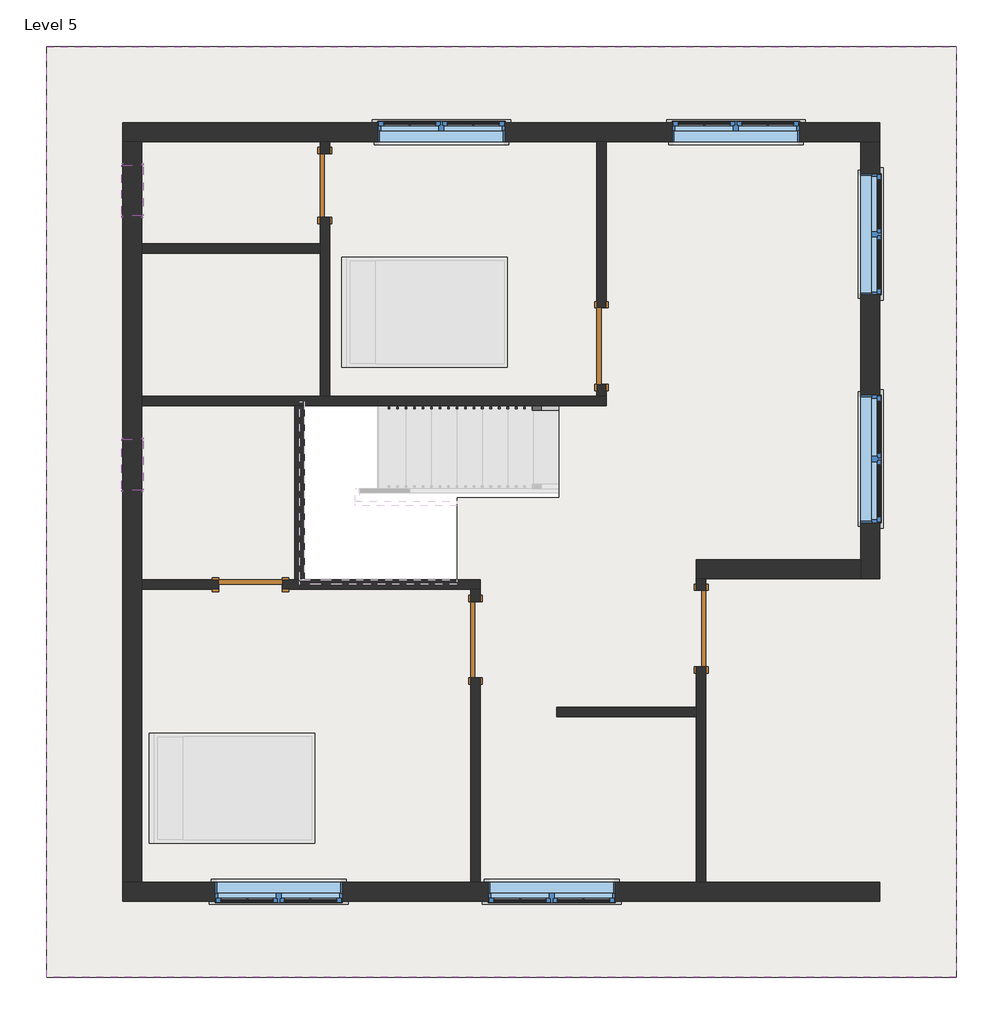
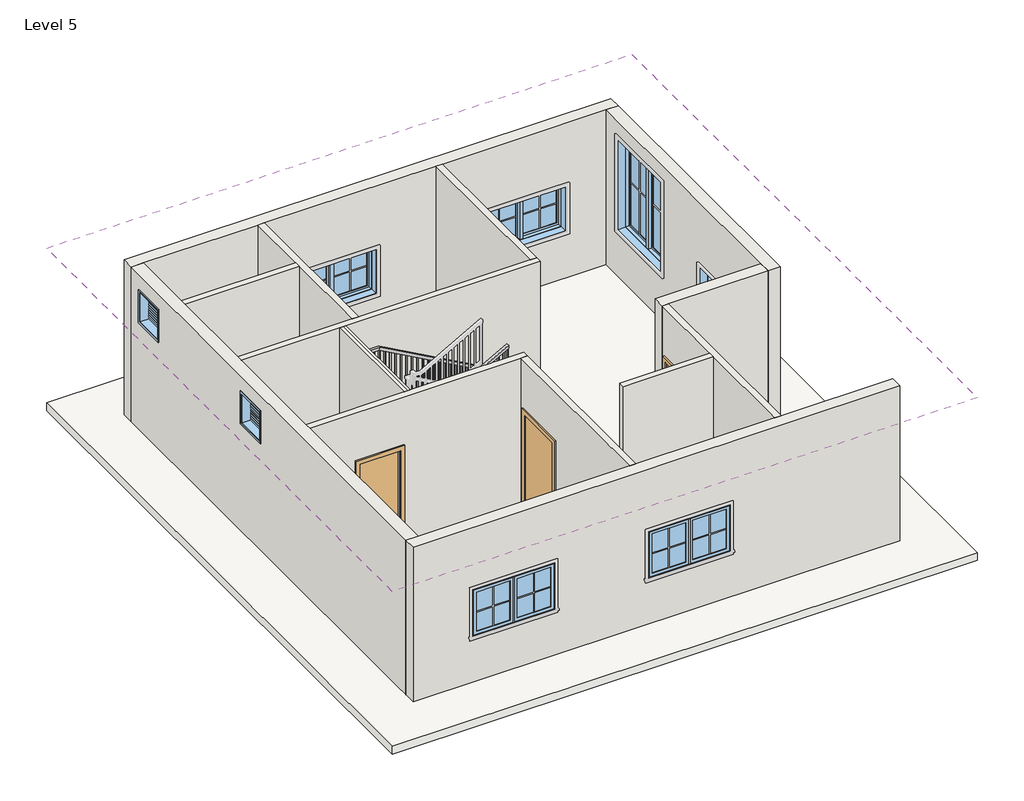
# One storey, part 1 of 2: 14 walls, 8 windows, 5 doors, 2 roofs, 1 railing.
"""IFC4 building model written with IfcOpenShell, lengths in millimetres."""

from ifc_helpers import new_model, si_unit, frame, origin, place, context, project, spatial, polyline, outline, extrude, faceted_brep, transform, mapped, element, save
from components import single_flush_3_17d80c48, single_flush_3_5e62189b, door_d8f5dbb5, window_9ac97e1a, window_c1d95f0f, window_f2d8fef0

model = new_model("IFC4")

# Units and contexts
model_context = context("Model", 3, world=origin())
ifc_project = project(units=[si_unit("LENGTHUNIT", "METRE", prefix="MILLI")], contexts=[model_context])

# Site, building, storey
site = spatial("IfcSite", under=ifc_project)
building = spatial("IfcBuilding", under=site)
storey = spatial("IfcBuildingStorey", under=building, Name="Level 5", Elevation=12649.2)

# Doors
placement = place(None, origin())
single_flush_3_shape = single_flush_3_17d80c48(model_context)
element("IfcDoor", 1, ObjectType="Single-Flush : 3'", at=placement, inside=storey, context=model_context, shape_type="MappedRepresentation", body=[
    mapped(single_flush_3_shape, transform((-1566.5130704, -2143.0042021, 12649.2), x_axis=(0.0, 1.0, 0.0), y_axis=(-1.0, 0.0, 0.0), z_axis=(0.0, 0.0, 1.0))),
])
single_flush_3_2_shape = single_flush_3_5e62189b(model_context)
element("IfcDoor", 2, ObjectType="Single-Flush : 3'", at=placement, inside=storey, context=model_context, shape_type="MappedRepresentation", body=[
    mapped(single_flush_3_2_shape, transform((1138.5869296, -2009.6542021, 12649.2), x_axis=(0.0, 1.0, 0.0), y_axis=(-1.0, 0.0, 0.0), z_axis=(0.0, 0.0, 1.0))),
])
element("IfcDoor", 3, ObjectType="Single-Flush : 3'", at=placement, inside=storey, context=model_context, shape_type="MappedRepresentation", body=[
    mapped(single_flush_3_2_shape, transform((-55.2130704, 1374.8957979, 12649.2), x_axis=(0.0, -1.0, 0.0), y_axis=(1.0, 0.0, 0.0), z_axis=(0.0, 0.0, 1.0))),
])
door_shape = door_d8f5dbb5(model_context)
element("IfcDoor", 4, ObjectType="Single-Flush : DOOR 2'6\"", at=placement, inside=storey, context=model_context, shape_type="MappedRepresentation", body=[
    mapped(door_shape, transform((-3369.9130704, 3298.9457979, 12649.2), x_axis=(0.0, 1.0, 0.0), y_axis=(-1.0, 0.0, 0.0), z_axis=(0.0, 0.0, 1.0))),
])
element("IfcDoor", 5, ObjectType="Single-Flush : DOOR 2'6\"", at=placement, inside=storey, context=model_context, shape_type="MappedRepresentation", body=[
    mapped(door_shape, transform((-4258.9130704, -1482.6042021, 12649.2), x_axis=(1.0, 0.0, 0.0), y_axis=(0.0, 1.0, 0.0), z_axis=(0.0, 0.0, 1.0))),
])

# Railing
element("IfcRailing", 6, ObjectType="Handrail - Rectangular", at=placement, inside=storey, context=model_context, shape_type="SolidModel", body=[
    faceted_brep([(-569.5630704, 606.5457979, 13732.9333333), (-569.5630704, 606.5457979, 13674.820221), (-569.5630704, 657.3457979, 13674.820221), (-569.5630704, 657.3457979, 13732.9333333), (-3007.9630704, 606.5457979, 15087.6), (-3021.1266727, 606.5457979, 15036.8), (-3021.1266727, 657.3457979, 15036.8), (-3007.9630704, 657.3457979, 15087.6), (-3566.7630704, 606.5457979, 15087.6), (-3566.7630704, 606.5457979, 15036.8), (-3617.5630704, 657.3457979, 15036.8), (-3617.5630704, 657.3457979, 15087.6), (-3566.7630704, -1374.6542021, 15087.6), (-3566.7630704, -1374.6542021, 15036.8), (-3617.5630704, -1425.4542021, 15036.8), (-3617.5630704, -1425.4542021, 15087.6), (-3312.7630704, -1374.6542021, 15087.6), (-3299.5994682, -1374.6542021, 15036.8), (-3299.5994682, -1425.4542021, 15036.8), (-3312.7630704, -1425.4542021, 15087.6), (-1788.7630704, -1374.6542021, 15934.2666667), (-1788.7630704, -1425.4542021, 15934.2666667), (-1788.7630704, -1425.4542021, 15876.1535543), (-1788.7630704, -1374.6542021, 15876.1535543)], [[[0, 1, 2, 3]], [[1, 0, 4, 5]], [[2, 1, 5, 6]], [[3, 2, 6, 7]], [[0, 3, 7, 4]], [[5, 4, 8, 9]], [[6, 5, 9, 10]], [[7, 6, 10, 11]], [[4, 7, 11, 8]], [[9, 8, 12, 13]], [[10, 9, 13, 14]], [[11, 10, 14, 15]], [[8, 11, 15, 12]], [[13, 12, 16, 17]], [[14, 13, 17, 18]], [[15, 14, 18, 19]], [[12, 15, 19, 16]], [[20, 21, 22, 23]], [[17, 16, 20, 23]], [[18, 17, 23, 22]], [[19, 18, 22, 21]], [[16, 19, 21, 20]]]),
    extrude(outline(polyline([(15839.1118876, -1855.4380704), (15828.5285543, -1874.4880704), (14850.5333333, -1874.4880704), (14850.5333333, -1855.4380704), (15839.1118876, -1855.4380704)])), frame((0.0, -1409.5792021, 0.0), z_axis=(0.0, 1.0, 0.0), x_axis=(0.0, 0.0, 1.0)), (0.0, 0.0, 1.0), 19.05),
    extrude(outline(polyline([(15782.6674432, -1957.0380704), (15772.0841099, -1976.0880704), (14850.5333333, -1976.0880704), (14850.5333333, -1957.0380704), (15782.6674432, -1957.0380704)])), frame((0.0, -1409.5792021, 0.0), z_axis=(0.0, 1.0, 0.0), x_axis=(0.0, 0.0, 1.0)), (0.0, 0.0, 1.0), 19.05),
    extrude(outline(polyline([(15726.2229988, -2058.6380704), (15715.6396654, -2077.6880704), (14850.5333333, -2077.6880704), (14850.5333333, -2058.6380704), (15726.2229988, -2058.6380704)])), frame((0.0, -1409.5792021, 0.0), z_axis=(0.0, 1.0, 0.0), x_axis=(0.0, 0.0, 1.0)), (0.0, 0.0, 1.0), 19.05),
    extrude(outline(polyline([(15669.7785543, -2160.2380704), (15659.195221, -2179.2880704), (14681.2, -2179.2880704), (14681.2, -2160.2380704), (15669.7785543, -2160.2380704)])), frame((0.0, -1409.5792021, 0.0), z_axis=(0.0, 1.0, 0.0), x_axis=(0.0, 0.0, 1.0)), (0.0, 0.0, 1.0), 19.05),
    extrude(outline(polyline([(15613.3341099, -2261.8380704), (15602.7507765, -2280.8880704), (14681.2, -2280.8880704), (14681.2, -2261.8380704), (15613.3341099, -2261.8380704)])), frame((0.0, -1409.5792021, 0.0), z_axis=(0.0, 1.0, 0.0), x_axis=(0.0, 0.0, 1.0)), (0.0, 0.0, 1.0), 19.05),
    extrude(outline(polyline([(15556.8896654, -2363.4380704), (15546.3063321, -2382.4880704), (14681.2, -2382.4880704), (14681.2, -2363.4380704), (15556.8896654, -2363.4380704)])), frame((0.0, -1409.5792021, 0.0), z_axis=(0.0, 1.0, 0.0), x_axis=(0.0, 0.0, 1.0)), (0.0, 0.0, 1.0), 19.05),
    extrude(outline(polyline([(15500.445221, -2465.0380704), (15489.8618876, -2484.0880704), (14511.8666667, -2484.0880704), (14511.8666667, -2465.0380704), (15500.445221, -2465.0380704)])), frame((0.0, -1409.5792021, 0.0), z_axis=(0.0, 1.0, 0.0), x_axis=(0.0, 0.0, 1.0)), (0.0, 0.0, 1.0), 19.05),
    extrude(outline(polyline([(15444.0007765, -2566.6380704), (15433.4174432, -2585.6880704), (14511.8666667, -2585.6880704), (14511.8666667, -2566.6380704), (15444.0007765, -2566.6380704)])), frame((0.0, -1409.5792021, 0.0), z_axis=(0.0, 1.0, 0.0), x_axis=(0.0, 0.0, 1.0)), (0.0, 0.0, 1.0), 19.05),
    extrude(outline(polyline([(15387.5563321, -2668.2380704), (15376.9729988, -2687.2880704), (14511.8666667, -2687.2880704), (14511.8666667, -2668.2380704), (15387.5563321, -2668.2380704)])), frame((0.0, -1409.5792021, 0.0), z_axis=(0.0, 1.0, 0.0), x_axis=(0.0, 0.0, 1.0)), (0.0, 0.0, 1.0), 19.05),
    extrude(outline(polyline([(15331.1118876, -2769.8380704), (15320.5285543, -2788.8880704), (14342.5333333, -2788.8880704), (14342.5333333, -2769.8380704), (15331.1118876, -2769.8380704)])), frame((0.0, -1409.5792021, 0.0), z_axis=(0.0, 1.0, 0.0), x_axis=(0.0, 0.0, 1.0)), (0.0, 0.0, 1.0), 19.05),
    extrude(outline(polyline([(15274.6674432, -2871.4380704), (15264.0841099, -2890.4880704), (14342.5333333, -2890.4880704), (14342.5333333, -2871.4380704), (15274.6674432, -2871.4380704)])), frame((0.0, -1409.5792021, 0.0), z_axis=(0.0, 1.0, 0.0), x_axis=(0.0, 0.0, 1.0)), (0.0, 0.0, 1.0), 19.05),
    extrude(outline(polyline([(15218.2229988, -2973.0380704), (15207.6396654, -2992.0880704), (14342.5333333, -2992.0880704), (14342.5333333, -2973.0380704), (15218.2229988, -2973.0380704)])), frame((0.0, -1409.5792021, 0.0), z_axis=(0.0, 1.0, 0.0), x_axis=(0.0, 0.0, 1.0)), (0.0, 0.0, 1.0), 19.05),
    extrude(outline(polyline([(15161.7785543, -3074.6380704), (15151.195221, -3093.6880704), (14173.2, -3093.6880704), (14173.2, -3074.6380704), (15161.7785543, -3074.6380704)])), frame((0.0, -1409.5792021, 0.0), z_axis=(0.0, 1.0, 0.0), x_axis=(0.0, 0.0, 1.0)), (0.0, 0.0, 1.0), 19.05),
    extrude(outline(polyline([(15105.3341099, -3176.2380704), (15094.7507765, -3195.2880704), (14173.2, -3195.2880704), (14173.2, -3176.2380704), (15105.3341099, -3176.2380704)])), frame((0.0, -1409.5792021, 0.0), z_axis=(0.0, 1.0, 0.0), x_axis=(0.0, 0.0, 1.0)), (0.0, 0.0, 1.0), 19.05),
    extrude(outline(polyline([(15048.8896654, -3277.8380704), (15038.3063321, -3296.8880704), (14173.2, -3296.8880704), (14173.2, -3277.8380704), (15048.8896654, -3277.8380704)])), frame((0.0, -1409.5792021, 0.0), z_axis=(0.0, 1.0, 0.0), x_axis=(0.0, 0.0, 1.0)), (0.0, 0.0, 1.0), 19.05),
    extrude(outline(polyline([(-3398.4880704, -1409.5792021), (-3398.4880704, -1390.5292021), (-3379.4380704, -1390.5292021), (-3379.4380704, -1409.5792021), (-3398.4880704, -1409.5792021)])), frame((0.0, 0.0, 14173.2), z_axis=(0.0, 0.0, 1.0), x_axis=(1.0, 0.0, 0.0)), (0.0, 0.0, 1.0), 863.6),
    extrude(outline(polyline([(-3500.0880704, -1409.5792021), (-3500.0880704, -1390.5292021), (-3481.0380704, -1390.5292021), (-3481.0380704, -1409.5792021), (-3500.0880704, -1409.5792021)])), frame((0.0, 0.0, 14173.2), z_axis=(0.0, 0.0, 1.0), x_axis=(1.0, 0.0, 0.0)), (0.0, 0.0, 1.0), 863.6),
    extrude(outline(polyline([(-3601.6880704, -1288.9292021), (-3582.6380704, -1288.9292021), (-3582.6380704, -1307.9792021), (-3601.6880704, -1307.9792021), (-3601.6880704, -1288.9292021)])), frame((0.0, 0.0, 14173.2), z_axis=(0.0, 0.0, 1.0), x_axis=(1.0, 0.0, 0.0)), (0.0, 0.0, 1.0), 863.6),
    extrude(outline(polyline([(-3601.6880704, -1187.3292021), (-3582.6380704, -1187.3292021), (-3582.6380704, -1206.3792021), (-3601.6880704, -1206.3792021), (-3601.6880704, -1187.3292021)])), frame((0.0, 0.0, 14173.2), z_axis=(0.0, 0.0, 1.0), x_axis=(1.0, 0.0, 0.0)), (0.0, 0.0, 1.0), 863.6),
    extrude(outline(polyline([(-3601.6880704, -1085.7292021), (-3582.6380704, -1085.7292021), (-3582.6380704, -1104.7792021), (-3601.6880704, -1104.7792021), (-3601.6880704, -1085.7292021)])), frame((0.0, 0.0, 14173.2), z_axis=(0.0, 0.0, 1.0), x_axis=(1.0, 0.0, 0.0)), (0.0, 0.0, 1.0), 863.6),
    extrude(outline(polyline([(-3601.6880704, -984.1292021), (-3582.6380704, -984.1292021), (-3582.6380704, -1003.1792021), (-3601.6880704, -1003.1792021), (-3601.6880704, -984.1292021)])), frame((0.0, 0.0, 14173.2), z_axis=(0.0, 0.0, 1.0), x_axis=(1.0, 0.0, 0.0)), (0.0, 0.0, 1.0), 863.6),
    extrude(outline(polyline([(-3601.6880704, -882.5292021), (-3582.6380704, -882.5292021), (-3582.6380704, -901.5792021), (-3601.6880704, -901.5792021), (-3601.6880704, -882.5292021)])), frame((0.0, 0.0, 14173.2), z_axis=(0.0, 0.0, 1.0), x_axis=(1.0, 0.0, 0.0)), (0.0, 0.0, 1.0), 863.6),
    extrude(outline(polyline([(-3601.6880704, -780.9292021), (-3582.6380704, -780.9292021), (-3582.6380704, -799.9792021), (-3601.6880704, -799.9792021), (-3601.6880704, -780.9292021)])), frame((0.0, 0.0, 14173.2), z_axis=(0.0, 0.0, 1.0), x_axis=(1.0, 0.0, 0.0)), (0.0, 0.0, 1.0), 863.6),
    extrude(outline(polyline([(-3601.6880704, -679.3292021), (-3582.6380704, -679.3292021), (-3582.6380704, -698.3792021), (-3601.6880704, -698.3792021), (-3601.6880704, -679.3292021)])), frame((0.0, 0.0, 14173.2), z_axis=(0.0, 0.0, 1.0), x_axis=(1.0, 0.0, 0.0)), (0.0, 0.0, 1.0), 863.6),
    extrude(outline(polyline([(-3601.6880704, -577.7292021), (-3582.6380704, -577.7292021), (-3582.6380704, -596.7792021), (-3601.6880704, -596.7792021), (-3601.6880704, -577.7292021)])), frame((0.0, 0.0, 14173.2), z_axis=(0.0, 0.0, 1.0), x_axis=(1.0, 0.0, 0.0)), (0.0, 0.0, 1.0), 863.6),
    extrude(outline(polyline([(-3601.6880704, -476.1292021), (-3582.6380704, -476.1292021), (-3582.6380704, -495.1792021), (-3601.6880704, -495.1792021), (-3601.6880704, -476.1292021)])), frame((0.0, 0.0, 14173.2), z_axis=(0.0, 0.0, 1.0), x_axis=(1.0, 0.0, 0.0)), (0.0, 0.0, 1.0), 863.6),
    extrude(outline(polyline([(-3601.6880704, -374.5292021), (-3582.6380704, -374.5292021), (-3582.6380704, -393.5792021), (-3601.6880704, -393.5792021), (-3601.6880704, -374.5292021)])), frame((0.0, 0.0, 14173.2), z_axis=(0.0, 0.0, 1.0), x_axis=(1.0, 0.0, 0.0)), (0.0, 0.0, 1.0), 863.6),
    extrude(outline(polyline([(-3601.6880704, -272.9292021), (-3582.6380704, -272.9292021), (-3582.6380704, -291.9792021), (-3601.6880704, -291.9792021), (-3601.6880704, -272.9292021)])), frame((0.0, 0.0, 14173.2), z_axis=(0.0, 0.0, 1.0), x_axis=(1.0, 0.0, 0.0)), (0.0, 0.0, 1.0), 863.6),
    extrude(outline(polyline([(-3601.6880704, -171.3292021), (-3582.6380704, -171.3292021), (-3582.6380704, -190.3792021), (-3601.6880704, -190.3792021), (-3601.6880704, -171.3292021)])), frame((0.0, 0.0, 14173.2), z_axis=(0.0, 0.0, 1.0), x_axis=(1.0, 0.0, 0.0)), (0.0, 0.0, 1.0), 863.6),
    extrude(outline(polyline([(-3601.6880704, -69.7292021), (-3582.6380704, -69.7292021), (-3582.6380704, -88.7792021), (-3601.6880704, -88.7792021), (-3601.6880704, -69.7292021)])), frame((0.0, 0.0, 14173.2), z_axis=(0.0, 0.0, 1.0), x_axis=(1.0, 0.0, 0.0)), (0.0, 0.0, 1.0), 863.6),
    extrude(outline(polyline([(-3601.6880704, 31.8707979), (-3582.6380704, 31.8707979), (-3582.6380704, 12.8207979), (-3601.6880704, 12.8207979), (-3601.6880704, 31.8707979)])), frame((0.0, 0.0, 14173.2), z_axis=(0.0, 0.0, 1.0), x_axis=(1.0, 0.0, 0.0)), (0.0, 0.0, 1.0), 863.6),
    extrude(outline(polyline([(-3601.6880704, 133.4707979), (-3582.6380704, 133.4707979), (-3582.6380704, 114.4207979), (-3601.6880704, 114.4207979), (-3601.6880704, 133.4707979)])), frame((0.0, 0.0, 14173.2), z_axis=(0.0, 0.0, 1.0), x_axis=(1.0, 0.0, 0.0)), (0.0, 0.0, 1.0), 863.6),
    extrude(outline(polyline([(-3601.6880704, 235.0707979), (-3582.6380704, 235.0707979), (-3582.6380704, 216.0207979), (-3601.6880704, 216.0207979), (-3601.6880704, 235.0707979)])), frame((0.0, 0.0, 14173.2), z_axis=(0.0, 0.0, 1.0), x_axis=(1.0, 0.0, 0.0)), (0.0, 0.0, 1.0), 863.6),
    extrude(outline(polyline([(-3601.6880704, 336.6707979), (-3582.6380704, 336.6707979), (-3582.6380704, 317.6207979), (-3601.6880704, 317.6207979), (-3601.6880704, 336.6707979)])), frame((0.0, 0.0, 14173.2), z_axis=(0.0, 0.0, 1.0), x_axis=(1.0, 0.0, 0.0)), (0.0, 0.0, 1.0), 863.6),
    extrude(outline(polyline([(-3601.6880704, 438.2707979), (-3582.6380704, 438.2707979), (-3582.6380704, 419.2207979), (-3601.6880704, 419.2207979), (-3601.6880704, 438.2707979)])), frame((0.0, 0.0, 14173.2), z_axis=(0.0, 0.0, 1.0), x_axis=(1.0, 0.0, 0.0)), (0.0, 0.0, 1.0), 863.6),
    extrude(outline(polyline([(-3601.6880704, 539.8707979), (-3582.6380704, 539.8707979), (-3582.6380704, 520.8207979), (-3601.6880704, 520.8207979), (-3601.6880704, 539.8707979)])), frame((0.0, 0.0, 14173.2), z_axis=(0.0, 0.0, 1.0), x_axis=(1.0, 0.0, 0.0)), (0.0, 0.0, 1.0), 863.6),
    extrude(outline(polyline([(-3506.4380704, 641.4707979), (-3506.4380704, 622.4207979), (-3525.4880704, 622.4207979), (-3525.4880704, 641.4707979), (-3506.4380704, 641.4707979)])), frame((0.0, 0.0, 14173.2), z_axis=(0.0, 0.0, 1.0), x_axis=(1.0, 0.0, 0.0)), (0.0, 0.0, 1.0), 863.6),
    extrude(outline(polyline([(-3404.8380704, 641.4707979), (-3404.8380704, 622.4207979), (-3423.8880704, 622.4207979), (-3423.8880704, 641.4707979), (-3404.8380704, 641.4707979)])), frame((0.0, 0.0, 14173.2), z_axis=(0.0, 0.0, 1.0), x_axis=(1.0, 0.0, 0.0)), (0.0, 0.0, 1.0), 863.6),
    extrude(outline(polyline([(-3303.2380704, 641.4707979), (-3303.2380704, 622.4207979), (-3322.2880704, 622.4207979), (-3322.2880704, 641.4707979), (-3303.2380704, 641.4707979)])), frame((0.0, 0.0, 14173.2), z_axis=(0.0, 0.0, 1.0), x_axis=(1.0, 0.0, 0.0)), (0.0, 0.0, 1.0), 863.6),
    extrude(outline(polyline([(-3201.6380704, 641.4707979), (-3201.6380704, 622.4207979), (-3220.6880704, 622.4207979), (-3220.6880704, 641.4707979), (-3201.6380704, 641.4707979)])), frame((0.0, 0.0, 14173.2), z_axis=(0.0, 0.0, 1.0), x_axis=(1.0, 0.0, 0.0)), (0.0, 0.0, 1.0), 863.6),
    extrude(outline(polyline([(-3100.0380704, 641.4707979), (-3100.0380704, 622.4207979), (-3119.0880704, 622.4207979), (-3119.0880704, 641.4707979), (-3100.0380704, 641.4707979)])), frame((0.0, 0.0, 14173.2), z_axis=(0.0, 0.0, 1.0), x_axis=(1.0, 0.0, 0.0)), (0.0, 0.0, 1.0), 863.6),
    extrude(outline(polyline([(15024.195221, -2998.4380704), (15034.7785543, -3017.4880704), (14173.2, -3017.4880704), (14173.2, -2998.4380704), (15024.195221, -2998.4380704)])), frame((0.0, 622.4207979, 0.0), z_axis=(0.0, 1.0, 0.0), x_axis=(0.0, 0.0, 1.0)), (0.0, 0.0, 1.0), 19.05),
    extrude(outline(polyline([(14967.7507765, -2896.8380704), (14978.3341099, -2915.8880704), (14003.8666667, -2915.8880704), (14003.8666667, -2896.8380704), (14967.7507765, -2896.8380704)])), frame((0.0, 622.4207979, 0.0), z_axis=(0.0, 1.0, 0.0), x_axis=(0.0, 0.0, 1.0)), (0.0, 0.0, 1.0), 19.05),
    extrude(outline(polyline([(14911.3063321, -2795.2380704), (14921.8896654, -2814.2880704), (14003.8666667, -2814.2880704), (14003.8666667, -2795.2380704), (14911.3063321, -2795.2380704)])), frame((0.0, 622.4207979, 0.0), z_axis=(0.0, 1.0, 0.0), x_axis=(0.0, 0.0, 1.0)), (0.0, 0.0, 1.0), 19.05),
    extrude(outline(polyline([(14854.8618876, -2693.6380704), (14865.445221, -2712.6880704), (14003.8666667, -2712.6880704), (14003.8666667, -2693.6380704), (14854.8618876, -2693.6380704)])), frame((0.0, 622.4207979, 0.0), z_axis=(0.0, 1.0, 0.0), x_axis=(0.0, 0.0, 1.0)), (0.0, 0.0, 1.0), 19.05),
    extrude(outline(polyline([(14798.4174432, -2592.0380704), (14809.0007765, -2611.0880704), (13834.5333333, -2611.0880704), (13834.5333333, -2592.0380704), (14798.4174432, -2592.0380704)])), frame((0.0, 622.4207979, 0.0), z_axis=(0.0, 1.0, 0.0), x_axis=(0.0, 0.0, 1.0)), (0.0, 0.0, 1.0), 19.05),
    extrude(outline(polyline([(14741.9729988, -2490.4380704), (14752.5563321, -2509.4880704), (13834.5333333, -2509.4880704), (13834.5333333, -2490.4380704), (14741.9729988, -2490.4380704)])), frame((0.0, 622.4207979, 0.0), z_axis=(0.0, 1.0, 0.0), x_axis=(0.0, 0.0, 1.0)), (0.0, 0.0, 1.0), 19.05),
    extrude(outline(polyline([(14685.5285543, -2388.8380704), (14696.1118876, -2407.8880704), (13834.5333333, -2407.8880704), (13834.5333333, -2388.8380704), (14685.5285543, -2388.8380704)])), frame((0.0, 622.4207979, 0.0), z_axis=(0.0, 1.0, 0.0), x_axis=(0.0, 0.0, 1.0)), (0.0, 0.0, 1.0), 19.05),
    extrude(outline(polyline([(14629.0841099, -2287.2380704), (14639.6674432, -2306.2880704), (13665.2, -2306.2880704), (13665.2, -2287.2380704), (14629.0841099, -2287.2380704)])), frame((0.0, 622.4207979, 0.0), z_axis=(0.0, 1.0, 0.0), x_axis=(0.0, 0.0, 1.0)), (0.0, 0.0, 1.0), 19.05),
    extrude(outline(polyline([(14572.6396654, -2185.6380704), (14583.2229988, -2204.6880704), (13665.2, -2204.6880704), (13665.2, -2185.6380704), (14572.6396654, -2185.6380704)])), frame((0.0, 622.4207979, 0.0), z_axis=(0.0, 1.0, 0.0), x_axis=(0.0, 0.0, 1.0)), (0.0, 0.0, 1.0), 19.05),
    extrude(outline(polyline([(14516.195221, -2084.0380704), (14526.7785543, -2103.0880704), (13665.2, -2103.0880704), (13665.2, -2084.0380704), (14516.195221, -2084.0380704)])), frame((0.0, 622.4207979, 0.0), z_axis=(0.0, 1.0, 0.0), x_axis=(0.0, 0.0, 1.0)), (0.0, 0.0, 1.0), 19.05),
    extrude(outline(polyline([(14459.7507765, -1982.4380704), (14470.3341099, -2001.4880704), (13495.8666667, -2001.4880704), (13495.8666667, -1982.4380704), (14459.7507765, -1982.4380704)])), frame((0.0, 622.4207979, 0.0), z_axis=(0.0, 1.0, 0.0), x_axis=(0.0, 0.0, 1.0)), (0.0, 0.0, 1.0), 19.05),
    extrude(outline(polyline([(14403.3063321, -1880.8380704), (14413.8896654, -1899.8880704), (13495.8666667, -1899.8880704), (13495.8666667, -1880.8380704), (14403.3063321, -1880.8380704)])), frame((0.0, 622.4207979, 0.0), z_axis=(0.0, 1.0, 0.0), x_axis=(0.0, 0.0, 1.0)), (0.0, 0.0, 1.0), 19.05),
    extrude(outline(polyline([(14346.8618876, -1779.2380704), (14357.445221, -1798.2880704), (13495.8666667, -1798.2880704), (13495.8666667, -1779.2380704), (14346.8618876, -1779.2380704)])), frame((0.0, 622.4207979, 0.0), z_axis=(0.0, 1.0, 0.0), x_axis=(0.0, 0.0, 1.0)), (0.0, 0.0, 1.0), 19.05),
    extrude(outline(polyline([(14290.4174432, -1677.6380704), (14301.0007765, -1696.6880704), (13326.5333333, -1696.6880704), (13326.5333333, -1677.6380704), (14290.4174432, -1677.6380704)])), frame((0.0, 622.4207979, 0.0), z_axis=(0.0, 1.0, 0.0), x_axis=(0.0, 0.0, 1.0)), (0.0, 0.0, 1.0), 19.05),
    extrude(outline(polyline([(14233.9729988, -1576.0380704), (14244.5563321, -1595.0880704), (13326.5333333, -1595.0880704), (13326.5333333, -1576.0380704), (14233.9729988, -1576.0380704)])), frame((0.0, 622.4207979, 0.0), z_axis=(0.0, 1.0, 0.0), x_axis=(0.0, 0.0, 1.0)), (0.0, 0.0, 1.0), 19.05),
    extrude(outline(polyline([(14177.5285543, -1474.4380704), (14188.1118876, -1493.4880704), (13326.5333333, -1493.4880704), (13326.5333333, -1474.4380704), (14177.5285543, -1474.4380704)])), frame((0.0, 622.4207979, 0.0), z_axis=(0.0, 1.0, 0.0), x_axis=(0.0, 0.0, 1.0)), (0.0, 0.0, 1.0), 19.05),
    extrude(outline(polyline([(14121.0841099, -1372.8380704), (14131.6674432, -1391.8880704), (13157.2, -1391.8880704), (13157.2, -1372.8380704), (14121.0841099, -1372.8380704)])), frame((0.0, 622.4207979, 0.0), z_axis=(0.0, 1.0, 0.0), x_axis=(0.0, 0.0, 1.0)), (0.0, 0.0, 1.0), 19.05),
    extrude(outline(polyline([(14064.6396654, -1271.2380704), (14075.2229988, -1290.2880704), (13157.2, -1290.2880704), (13157.2, -1271.2380704), (14064.6396654, -1271.2380704)])), frame((0.0, 622.4207979, 0.0), z_axis=(0.0, 1.0, 0.0), x_axis=(0.0, 0.0, 1.0)), (0.0, 0.0, 1.0), 19.05),
    extrude(outline(polyline([(14008.195221, -1169.6380704), (14018.7785543, -1188.6880704), (13157.2, -1188.6880704), (13157.2, -1169.6380704), (14008.195221, -1169.6380704)])), frame((0.0, 622.4207979, 0.0), z_axis=(0.0, 1.0, 0.0), x_axis=(0.0, 0.0, 1.0)), (0.0, 0.0, 1.0), 19.05),
    extrude(outline(polyline([(13951.7507765, -1068.0380704), (13962.3341099, -1087.0880704), (12987.8666667, -1087.0880704), (12987.8666667, -1068.0380704), (13951.7507765, -1068.0380704)])), frame((0.0, 622.4207979, 0.0), z_axis=(0.0, 1.0, 0.0), x_axis=(0.0, 0.0, 1.0)), (0.0, 0.0, 1.0), 19.05),
    extrude(outline(polyline([(13895.3063321, -966.4380704), (13905.8896654, -985.4880704), (12987.8666667, -985.4880704), (12987.8666667, -966.4380704), (13895.3063321, -966.4380704)])), frame((0.0, 622.4207979, 0.0), z_axis=(0.0, 1.0, 0.0), x_axis=(0.0, 0.0, 1.0)), (0.0, 0.0, 1.0), 19.05),
    extrude(outline(polyline([(13838.8618876, -864.8380704), (13849.445221, -883.8880704), (12987.8666667, -883.8880704), (12987.8666667, -864.8380704), (13838.8618876, -864.8380704)])), frame((0.0, 622.4207979, 0.0), z_axis=(0.0, 1.0, 0.0), x_axis=(0.0, 0.0, 1.0)), (0.0, 0.0, 1.0), 19.05),
    extrude(outline(polyline([(13782.4174432, -763.2380704), (13793.0007765, -782.2880704), (12818.5333333, -782.2880704), (12818.5333333, -763.2380704), (13782.4174432, -763.2380704)])), frame((0.0, 622.4207979, 0.0), z_axis=(0.0, 1.0, 0.0), x_axis=(0.0, 0.0, 1.0)), (0.0, 0.0, 1.0), 19.05),
    extrude(outline(polyline([(13725.9729988, -661.6380704), (13736.5563321, -680.6880704), (12818.5333333, -680.6880704), (12818.5333333, -661.6380704), (13725.9729988, -661.6380704)])), frame((0.0, 622.4207979, 0.0), z_axis=(0.0, 1.0, 0.0), x_axis=(0.0, 0.0, 1.0)), (0.0, 0.0, 1.0), 19.05),
    extrude(outline(polyline([(-3601.6880704, -1390.5292021), (-3582.6380704, -1390.5292021), (-3582.6380704, -1409.5792021), (-3601.6880704, -1409.5792021), (-3601.6880704, -1390.5292021)])), frame((0.0, 0.0, 14173.2), z_axis=(0.0, 0.0, 1.0), x_axis=(1.0, 0.0, 0.0)), (0.0, 0.0, 1.0), 863.6),
    extrude(outline(polyline([(-3582.6380704, 641.4707979), (-3582.6380704, 622.4207979), (-3601.6880704, 622.4207979), (-3601.6880704, 641.4707979), (-3582.6380704, 641.4707979)])), frame((0.0, 0.0, 14173.2), z_axis=(0.0, 0.0, 1.0), x_axis=(1.0, 0.0, 0.0)), (0.0, 0.0, 1.0), 863.6),
    extrude(outline(polyline([(15876.1535543, -1788.7630704), (15865.570221, -1807.8130704), (14850.5333333, -1807.8130704), (14850.5333333, -1788.7630704), (15876.1535543, -1788.7630704)])), frame((0.0, -1409.5792021, 0.0), z_axis=(0.0, 1.0, 0.0), x_axis=(0.0, 0.0, 1.0)), (0.0, 0.0, 1.0), 19.05),
    extrude(outline(polyline([(13674.820221, -569.5630704), (13685.4035543, -588.6130704), (12818.5333333, -588.6130704), (12818.5333333, -569.5630704), (13674.820221, -569.5630704)])), frame((0.0, 622.4207979, 0.0), z_axis=(0.0, 1.0, 0.0), x_axis=(0.0, 0.0, 1.0)), (0.0, 0.0, 1.0), 19.05),
])

# Roofs
element("IfcRoof", 7, ObjectType="roof 6\"", at=placement, inside=storey, context=model_context, shape_type="SweptSolid", body=[
    extrude(outline(polyline([(4192.9369296, 4962.6457979), (4192.9369296, -6187.9542021), (-6703.6630704, -6187.9542021), (-6703.6630704, 4962.6457979), (4192.9369296, 4962.6457979)]), holes=[polyline([(-3668.3630704, 708.1457979), (-3668.3630704, -1476.2542021), (-1788.7630704, -1476.2542021), (-1788.7630704, -434.8542021), (-569.5630704, -434.8542021), (-569.5630704, 708.1457979), (-3668.3630704, 708.1457979)])]), frame((0.0, 0.0, 12496.8), z_axis=(0.0, 0.0, 1.0), x_axis=(1.0, 0.0, 0.0)), (0.0, 0.0, 1.0), 152.4),
])
element("IfcRoof", 8, ObjectType="roof 6\"", at=placement, inside=storey, context=model_context, shape_type="SweptSolid", body=[
    extrude(outline(polyline([(4192.9369296, 4962.6457979), (4192.9369296, -6187.9542021), (-6703.6630704, -6187.9542021), (-6703.6630704, 4962.6457979), (4192.9369296, 4962.6457979)]), holes=[polyline([(-3668.3630704, 708.1457979), (-3668.3630704, -1476.2542021), (-1788.7630704, -1476.2542021), (-1788.7630704, -434.8542021), (-569.5630704, -434.8542021), (-569.5630704, 708.1457979), (-3668.3630704, 708.1457979)])]), frame((0.0, 0.0, 15697.2), z_axis=(0.0, 0.0, 1.0), x_axis=(1.0, 0.0, 0.0)), (0.0, 0.0, 1.0), 152.4),
])

# Walls
element("IfcWall", 9, ObjectType="WALL 4.5\"", at=placement, inside=storey, context=model_context, shape_type="Brep", body=[
    faceted_brep([(-3427.0630704, 3819.6457979, 12649.2), (-3427.0630704, 3679.9457979, 12649.2), (-3427.0630704, 3679.9457979, 14681.2), (-3427.0630704, 2917.9457979, 14681.2), (-3427.0630704, 2917.9457979, 12649.2), (-3427.0630704, 2600.4457979, 12649.2), (-3427.0630704, 2486.1457979, 12649.2), (-3427.0630704, 771.6457979, 12649.2), (-3427.0630704, 771.6457979, 15697.2), (-3427.0630704, 2486.1457979, 15697.2), (-3427.0630704, 2600.4457979, 15697.2), (-3427.0630704, 3819.6457979, 15697.2), (-3312.7630704, 3679.9457979, 14681.2), (-3312.7630704, 3679.9457979, 12649.2), (-3312.7630704, 3819.6457979, 12649.2), (-3312.7630704, 3819.6457979, 15697.2), (-3312.7630704, 771.6457979, 15697.2), (-3312.7630704, 771.6457979, 12649.2), (-3312.7630704, 2917.9457979, 12649.2), (-3312.7630704, 2917.9457979, 14681.2)], [[[0, 1, 2, 3, 4, 5, 6, 7, 8, 9, 10, 11]], [[12, 13, 14, 15, 16, 17, 18, 19]], [[18, 17, 7, 6, 5, 4]], [[14, 13, 1, 0]], [[0, 11, 15, 14]], [[8, 7, 17, 16]], [[2, 1, 13, 12]], [[3, 2, 12, 19]], [[4, 3, 19, 18]], [[11, 10, 9, 8, 16, 15]]]),
])
element("IfcWall", 10, ObjectType="WALL 4.5\"", at=placement, inside=storey, context=model_context, shape_type="Brep", body=[
    faceted_brep([(-5560.6630704, 657.3457979, 12649.2), (-3731.8630704, 657.3457979, 12649.2), (-3617.5630704, 657.3457979, 12649.2), (1.9369296, 657.3457979, 12649.2), (1.9369296, 657.3457979, 15697.2), (-3617.5630704, 657.3457979, 15697.2), (-3731.8630704, 657.3457979, 15697.2), (-5560.6630704, 657.3457979, 15697.2), (-5560.6630704, 771.6457979, 12649.2), (-5560.6630704, 771.6457979, 15697.2), (-3427.0630704, 771.6457979, 15697.2), (-3312.7630704, 771.6457979, 15697.2), (-112.3630704, 771.6457979, 15697.2), (1.9369296, 771.6457979, 15697.2), (1.9369296, 771.6457979, 12649.2), (-112.3630704, 771.6457979, 12649.2), (-3312.7630704, 771.6457979, 12649.2), (-3427.0630704, 771.6457979, 12649.2)], [[[0, 1, 2, 3, 4, 5, 6, 7]], [[8, 9, 10, 11, 12, 13, 14, 15, 16, 17]], [[3, 2, 1, 0, 8, 17, 16, 15, 14]], [[7, 6, 5, 4, 13, 12, 11, 10, 9]], [[0, 7, 9, 8]], [[4, 3, 14, 13]]]),
])
element("IfcWall", 11, ObjectType="WALL 4.5\"", at=placement, inside=storey, context=model_context, shape_type="SweptSolid", body=[
    extrude(outline(polyline([(917.6957979, 14681.2), (917.6957979, 12649.2), (771.6457979, 12649.2), (771.6457979, 15697.2), (3819.6457979, 15697.2), (3819.6457979, 12649.2), (1832.0957979, 12649.2), (1832.0957979, 14681.2), (917.6957979, 14681.2)])), frame((-112.3630704, 0.0, 0.0), z_axis=(1.0, 0.0, 0.0), x_axis=(0.0, 1.0, 0.0)), (0.0, 0.0, 1.0), 114.3),
])
element("IfcWall", 12, ObjectType="WALL 4.5\"", at=placement, inside=storey, context=model_context, shape_type="SweptSolid", body=[
    extrude(outline(polyline([(-3427.0630704, 2486.1457979), (-5560.6630704, 2486.1457979), (-5560.6630704, 2600.4457979), (-3427.0630704, 2600.4457979), (-3427.0630704, 2486.1457979)])), frame((0.0, 0.0, 12649.2), z_axis=(0.0, 0.0, 1.0), x_axis=(1.0, 0.0, 0.0)), (0.0, 0.0, 1.0), 3048.0),
])
element("IfcWall", 13, ObjectType="WALL 4.5\"", at=placement, inside=storey, context=model_context, shape_type="Brep", body=[
    faceted_brep([(-3877.9130704, -1539.7542021, 14681.2), (-3877.9130704, -1539.7542021, 12649.2), (-1623.6630704, -1539.7542021, 12649.2), (-1509.3630704, -1539.7542021, 12649.2), (-1509.3630704, -1539.7542021, 15697.2), (-1623.6630704, -1539.7542021, 15697.2), (-5560.6630704, -1539.7542021, 15697.2), (-5560.6630704, -1539.7542021, 12649.2), (-4639.9130704, -1539.7542021, 12649.2), (-4639.9130704, -1539.7542021, 14681.2), (-1509.3630704, -1425.4542021, 12649.2), (-3617.5630704, -1425.4542021, 12649.2), (-3731.8630704, -1425.4542021, 12649.2), (-3877.9130704, -1425.4542021, 12649.2), (-3877.9130704, -1425.4542021, 14681.2), (-4639.9130704, -1425.4542021, 14681.2), (-4639.9130704, -1425.4542021, 12649.2), (-5560.6630704, -1425.4542021, 12649.2), (-5560.6630704, -1425.4542021, 15697.2), (-3731.8630704, -1425.4542021, 15697.2), (-3617.5630704, -1425.4542021, 15697.2), (-1509.3630704, -1425.4542021, 15697.2)], [[[0, 1, 2, 3, 4, 5, 6, 7, 8, 9]], [[10, 11, 12, 13, 14, 15, 16, 17, 18, 19, 20, 21]], [[8, 7, 17, 16]], [[3, 2, 1, 13, 12, 11, 10]], [[6, 5, 4, 21, 20, 19, 18]], [[7, 6, 18, 17]], [[4, 3, 10, 21]], [[14, 13, 1, 0]], [[15, 14, 0, 9]], [[16, 15, 9, 8]]]),
])
element("IfcWall", 14, ObjectType="WALL 4.5\"", at=placement, inside=storey, context=model_context, shape_type="SweptSolid", body=[
    extrude(outline(polyline([(-1539.7542021, 12649.2), (-1685.8042021, 12649.2), (-1685.8042021, 14681.2), (-2600.2042021, 14681.2), (-2600.2042021, 12649.2), (-5044.9542021, 12649.2), (-5044.9542021, 15697.2), (-1539.7542021, 15697.2), (-1539.7542021, 12649.2)])), frame((-1623.6630704, 0.0, 0.0), z_axis=(1.0, 0.0, 0.0), x_axis=(0.0, 1.0, 0.0)), (0.0, 0.0, 1.0), 114.3),
])
element("IfcWall", 15, ObjectType="WALL 4.5\"", at=placement, inside=storey, context=model_context, shape_type="Brep", body=[
    faceted_brep([(1195.7369296, -1552.4542021, 14681.2), (1195.7369296, -1552.4542021, 12649.2), (1195.7369296, -1412.7542021, 12649.2), (1195.7369296, -1412.7542021, 15697.2), (1195.7369296, -5044.9542021, 15697.2), (1195.7369296, -5044.9542021, 12649.2), (1195.7369296, -2466.8542021, 12649.2), (1195.7369296, -2466.8542021, 14681.2), (1081.4369296, -1412.7542021, 12649.2), (1081.4369296, -1552.4542021, 12649.2), (1081.4369296, -1552.4542021, 14681.2), (1081.4369296, -2466.8542021, 14681.2), (1081.4369296, -2466.8542021, 12649.2), (1081.4369296, -2948.9967683, 12649.2), (1081.4369296, -3063.2967683, 12649.2), (1081.4369296, -5044.9542021, 12649.2), (1081.4369296, -5044.9542021, 15697.2), (1081.4369296, -3063.2967683, 15697.2), (1081.4369296, -2948.9967683, 15697.2), (1081.4369296, -1412.7542021, 15697.2)], [[[0, 1, 2, 3, 4, 5, 6, 7]], [[8, 9, 10, 11, 12, 13, 14, 15, 16, 17, 18, 19]], [[6, 5, 15, 14, 13, 12]], [[2, 1, 9, 8]], [[3, 2, 8, 19]], [[5, 4, 16, 15]], [[10, 9, 1, 0]], [[11, 10, 0, 7]], [[12, 11, 7, 6]], [[4, 3, 19, 18, 17, 16]]]),
])
element("IfcWall", 16, ObjectType="WALL 4.5\"", at=placement, inside=storey, context=model_context, shape_type="SweptSolid", body=[
    extrude(outline(polyline([(-594.9630704, -2948.9967683), (1081.4369296, -2948.9967683), (1081.4369296, -3063.2967683), (-594.9630704, -3063.2967683), (-594.9630704, -2948.9967683)])), frame((0.0, 0.0, 12649.2), z_axis=(0.0, 0.0, 1.0), x_axis=(1.0, 0.0, 0.0)), (0.0, 0.0, 1.0), 3048.0),
])
element("IfcWall", 17, ObjectType="WALL 4.5\"", at=placement, inside=storey, context=model_context, shape_type="SweptSolid", body=[
    extrude(outline(polyline([(15697.2, -3731.8630704), (12649.2, -3731.8630704), (12649.2, -3617.5630704), (15697.2, -3617.5630704), (15697.2, -3668.3630704), (15697.2, -3731.8630704)])), frame((0.0, -1425.4542021, 0.0), z_axis=(0.0, 1.0, 0.0), x_axis=(0.0, 0.0, 1.0)), (0.0, 0.0, 1.0), 2082.8),
])
element("IfcWall", 18, ObjectType="WALL 9\"", at=placement, inside=storey, context=model_context, shape_type="Brep", body=[
    faceted_brep([(-5789.2630704, 3819.6457979, 12649.2), (-5560.6630704, 3819.6457979, 12649.2), (-3427.0630704, 3819.6457979, 12649.2), (-3312.7630704, 3819.6457979, 12649.2), (-112.3630704, 3819.6457979, 12649.2), (1.9369296, 3819.6457979, 12649.2), (3049.9369296, 3819.6457979, 12649.2), (3278.5369296, 3819.6457979, 12649.2), (3278.5369296, 3819.6457979, 15697.2), (3049.9369296, 3819.6457979, 15697.2), (1.9369296, 3819.6457979, 15697.2), (-112.3630704, 3819.6457979, 15697.2), (-3312.7630704, 3819.6457979, 15697.2), (-3427.0630704, 3819.6457979, 15697.2), (-5560.6630704, 3819.6457979, 15697.2), (-5789.2630704, 3819.6457979, 15697.2), (2316.5119296, 3819.6457979, 14478.0), (2316.5119296, 3819.6457979, 13563.6), (792.5119296, 3819.6457979, 13563.6), (792.5119296, 3819.6457979, 14478.0), (-1210.9130704, 3819.6457979, 14478.0), (-1210.9130704, 3819.6457979, 13563.6), (-2734.9130704, 3819.6457979, 13563.6), (-2734.9130704, 3819.6457979, 14478.0), (-5789.2630704, 4048.2457979, 12649.2), (-5789.2630704, 4048.2457979, 15697.2), (3278.5369296, 4048.2457979, 15697.2), (3278.5369296, 4048.2457979, 12649.2), (2316.5119296, 4048.2457979, 14478.0), (792.5119296, 4048.2457979, 14478.0), (792.5119296, 4048.2457979, 13563.6), (2316.5119296, 4048.2457979, 13563.6), (-1210.9130704, 4048.2457979, 14478.0), (-2734.9130704, 4048.2457979, 14478.0), (-2734.9130704, 4048.2457979, 13563.6), (-1210.9130704, 4048.2457979, 13563.6)], [[[0, 1, 2, 3, 4, 5, 6, 7, 8, 9, 10, 11, 12, 13, 14, 15], [16, 17, 18, 19], [20, 21, 22, 23]], [[24, 25, 26, 27], [28, 29, 30, 31], [32, 33, 34, 35]], [[7, 6, 5, 4, 3, 2, 1, 0, 24, 27]], [[8, 7, 27, 26]], [[0, 15, 25, 24]], [[17, 16, 28, 31]], [[18, 17, 31, 30]], [[19, 18, 30, 29]], [[16, 19, 29, 28]], [[21, 20, 32, 35]], [[22, 21, 35, 34]], [[23, 22, 34, 33]], [[20, 23, 33, 32]], [[15, 14, 13, 12, 11, 10, 9, 8, 26, 25]]]),
])
element("IfcWall", 19, ObjectType="WALL 9\"", at=placement, inside=storey, context=model_context, shape_type="Brep", body=[
    faceted_brep([(3049.9369296, 3819.6457979, 12649.2), (3049.9369296, -1184.1542021, 12649.2), (3049.9369296, -1412.7542021, 12649.2), (3049.9369296, -1412.7542021, 15697.2), (3049.9369296, -1184.1542021, 15697.2), (3049.9369296, 3819.6457979, 15697.2), (3049.9369296, -739.6542021, 14478.0), (3049.9369296, -739.6542021, 13563.6), (3049.9369296, 784.3457979, 13563.6), (3049.9369296, 784.3457979, 14478.0), (3049.9369296, 1990.8457979, 15392.4), (3049.9369296, 1990.8457979, 13563.6), (3049.9369296, 3438.6457979, 13563.6), (3049.9369296, 3438.6457979, 15392.4), (3278.5369296, 3819.6457979, 12649.2), (3278.5369296, 3819.6457979, 15697.2), (3278.5369296, -1412.7542021, 15697.2), (3278.5369296, -1412.7542021, 12649.2), (3278.5369296, -739.6542021, 14478.0), (3278.5369296, 784.3457979, 14478.0), (3278.5369296, 784.3457979, 13563.6), (3278.5369296, -739.6542021, 13563.6), (3278.5369296, 1990.8457979, 15392.4), (3278.5369296, 3438.6457979, 15392.4), (3278.5369296, 3438.6457979, 13563.6), (3278.5369296, 1990.8457979, 13563.6)], [[[0, 1, 2, 3, 4, 5], [6, 7, 8, 9], [10, 11, 12, 13]], [[14, 15, 16, 17], [18, 19, 20, 21], [22, 23, 24, 25]], [[2, 1, 0, 14, 17]], [[0, 5, 15, 14]], [[3, 2, 17, 16]], [[7, 6, 18, 21]], [[8, 7, 21, 20]], [[9, 8, 20, 19]], [[6, 9, 19, 18]], [[11, 10, 22, 25]], [[12, 11, 25, 24]], [[13, 12, 24, 23]], [[10, 13, 23, 22]], [[5, 4, 3, 16, 15]]]),
])
element("IfcWall", 20, ObjectType="WALL 9\"", at=placement, inside=storey, context=model_context, shape_type="Brep", body=[
    faceted_brep([(3049.9369296, -1184.1542021, 12649.2), (1081.4369296, -1184.1542021, 12649.2), (1081.4369296, -1184.1542021, 15697.2), (3049.9369296, -1184.1542021, 15697.2), (3049.9369296, -1412.7542021, 12649.2), (3049.9369296, -1412.7542021, 15697.2), (1195.7369296, -1412.7542021, 15697.2), (1081.4369296, -1412.7542021, 15697.2), (1081.4369296, -1412.7542021, 12649.2), (1195.7369296, -1412.7542021, 12649.2)], [[[0, 1, 2, 3]], [[4, 5, 6, 7, 8, 9]], [[1, 0, 4, 9, 8]], [[0, 3, 5, 4]], [[2, 1, 8, 7]], [[3, 2, 7, 6, 5]]]),
])
element("IfcWall", 21, ObjectType="WALL 9\"", at=placement, inside=storey, context=model_context, shape_type="Brep", body=[
    faceted_brep([(3278.5369296, -5044.9542021, 12649.2), (1195.7369296, -5044.9542021, 12649.2), (1081.4369296, -5044.9542021, 12649.2), (-1509.3630704, -5044.9542021, 12649.2), (-1623.6630704, -5044.9542021, 12649.2), (-5560.6630704, -5044.9542021, 12649.2), (-5789.2630704, -5044.9542021, 12649.2), (-5789.2630704, -5044.9542021, 15697.2), (-5560.6630704, -5044.9542021, 15697.2), (-1623.6630704, -5044.9542021, 15697.2), (-1509.3630704, -5044.9542021, 15697.2), (1081.4369296, -5044.9542021, 15697.2), (1195.7369296, -5044.9542021, 15697.2), (3278.5369296, -5044.9542021, 15697.2), (-4684.3630704, -5044.9542021, 14478.0), (-4684.3630704, -5044.9542021, 13563.6), (-3160.3630704, -5044.9542021, 13563.6), (-3160.3630704, -5044.9542021, 14478.0), (-1414.1130704, -5044.9542021, 14478.0), (-1414.1130704, -5044.9542021, 13563.6), (109.8869296, -5044.9542021, 13563.6), (109.8869296, -5044.9542021, 14478.0), (3278.5369296, -5273.5542021, 12649.2), (3278.5369296, -5273.5542021, 15697.2), (-5789.2630704, -5273.5542021, 15697.2), (-5789.2630704, -5273.5542021, 12649.2), (-4684.3630704, -5273.5542021, 14478.0), (-3160.3630704, -5273.5542021, 14478.0), (-3160.3630704, -5273.5542021, 13563.6), (-4684.3630704, -5273.5542021, 13563.6), (-1414.1130704, -5273.5542021, 14478.0), (109.8869296, -5273.5542021, 14478.0), (109.8869296, -5273.5542021, 13563.6), (-1414.1130704, -5273.5542021, 13563.6)], [[[0, 1, 2, 3, 4, 5, 6, 7, 8, 9, 10, 11, 12, 13], [14, 15, 16, 17], [18, 19, 20, 21]], [[22, 23, 24, 25], [26, 27, 28, 29], [30, 31, 32, 33]], [[6, 5, 4, 3, 2, 1, 0, 22, 25]], [[0, 13, 23, 22]], [[7, 6, 25, 24]], [[15, 14, 26, 29]], [[16, 15, 29, 28]], [[17, 16, 28, 27]], [[14, 17, 27, 26]], [[19, 18, 30, 33]], [[20, 19, 33, 32]], [[21, 20, 32, 31]], [[18, 21, 31, 30]], [[13, 12, 11, 10, 9, 8, 7, 24, 23]]]),
])
element("IfcWall", 22, ObjectType="WALL 9\"", at=placement, inside=storey, context=model_context, shape_type="Brep", body=[
    faceted_brep([(-5560.6630704, -5044.9542021, 12649.2), (-5560.6630704, -1539.7542021, 12649.2), (-5560.6630704, -1425.4542021, 12649.2), (-5560.6630704, 657.3457979, 12649.2), (-5560.6630704, 771.6457979, 12649.2), (-5560.6630704, 2486.1457979, 12649.2), (-5560.6630704, 2600.4457979, 12649.2), (-5560.6630704, 3819.6457979, 12649.2), (-5560.6630704, 3819.6457979, 15697.2), (-5560.6630704, 2600.4457979, 15697.2), (-5560.6630704, 2486.1457979, 15697.2), (-5560.6630704, 771.6457979, 15697.2), (-5560.6630704, 657.3457979, 15697.2), (-5560.6630704, -1425.4542021, 15697.2), (-5560.6630704, -1539.7542021, 15697.2), (-5560.6630704, -5044.9542021, 15697.2), (-5560.6630704, 257.2957979, 15392.4), (-5560.6630704, 257.2957979, 14782.8), (-5560.6630704, -352.3042021, 14782.8), (-5560.6630704, -352.3042021, 15392.4), (-5560.6630704, 3543.4207979, 15392.4), (-5560.6630704, 3543.4207979, 14782.8), (-5560.6630704, 2933.8207979, 14782.8), (-5560.6630704, 2933.8207979, 15392.4), (-5789.2630704, -5044.9542021, 12649.2), (-5789.2630704, -5044.9542021, 15697.2), (-5789.2630704, 3819.6457979, 15697.2), (-5789.2630704, 3819.6457979, 12649.2), (-5789.2630704, 257.2957979, 15392.4), (-5789.2630704, -352.3042021, 15392.4), (-5789.2630704, -352.3042021, 14782.8), (-5789.2630704, 257.2957979, 14782.8), (-5789.2630704, 3543.4207979, 15392.4), (-5789.2630704, 2933.8207979, 15392.4), (-5789.2630704, 2933.8207979, 14782.8), (-5789.2630704, 3543.4207979, 14782.8)], [[[0, 1, 2, 3, 4, 5, 6, 7, 8, 9, 10, 11, 12, 13, 14, 15], [16, 17, 18, 19], [20, 21, 22, 23]], [[24, 25, 26, 27], [28, 29, 30, 31], [32, 33, 34, 35]], [[7, 6, 5, 4, 3, 2, 1, 0, 24, 27]], [[0, 15, 25, 24]], [[8, 7, 27, 26]], [[17, 16, 28, 31]], [[18, 17, 31, 30]], [[19, 18, 30, 29]], [[16, 19, 29, 28]], [[21, 20, 32, 35]], [[22, 21, 35, 34]], [[23, 22, 34, 33]], [[20, 23, 33, 32]], [[15, 14, 13, 12, 11, 10, 9, 8, 26, 25]]]),
])

# Windows
window_shape = window_9ac97e1a(model_context)
element("IfcWindow", 23, ObjectType="Window-Casement-Double : 57\" x 72\"", at=placement, inside=storey, context=model_context, shape_type="MappedRepresentation", body=[
    mapped(window_shape, transform((3164.2369296, 2714.7457979, 12649.2), x_axis=(0.0, -1.0, 0.0), y_axis=(1.0, 0.0, 0.0), z_axis=(0.0, 0.0, 1.0))),
])
window_2_shape = window_c1d95f0f(model_context)
element("IfcWindow", 24, ObjectType="Window-Casement-Double : WINDOW 6\"", at=placement, inside=storey, context=model_context, shape_type="MappedRepresentation", body=[
    mapped(window_2_shape, transform((-3922.3630704, -5159.2542021, 12649.2), x_axis=(-1.0, 0.0, 0.0), y_axis=(0.0, -1.0, 0.0), z_axis=(0.0, 0.0, 1.0))),
])
element("IfcWindow", 25, ObjectType="Window-Casement-Double : WINDOW 6\"", at=placement, inside=storey, context=model_context, shape_type="MappedRepresentation", body=[
    mapped(window_2_shape, transform((-652.1130704, -5159.2542021, 12649.2), x_axis=(-1.0, 0.0, 0.0), y_axis=(0.0, -1.0, 0.0), z_axis=(0.0, 0.0, 1.0))),
])
element("IfcWindow", 26, ObjectType="Window-Casement-Double : WINDOW 6\"", at=placement, inside=storey, context=model_context, shape_type="MappedRepresentation", body=[
    mapped(window_2_shape, transform((3164.2369296, 22.3457979, 12649.2), x_axis=(0.0, -1.0, 0.0), y_axis=(1.0, 0.0, 0.0), z_axis=(0.0, 0.0, 1.0))),
])
element("IfcWindow", 27, ObjectType="Window-Casement-Double : WINDOW 6\"", at=placement, inside=storey, context=model_context, shape_type="MappedRepresentation", body=[
    mapped(window_2_shape, transform((1554.5119296, 3933.9457979, 12649.2), x_axis=(1.0, 0.0, 0.0), y_axis=(0.0, 1.0, 0.0), z_axis=(0.0, 0.0, 1.0))),
])
element("IfcWindow", 28, ObjectType="Window-Casement-Double : WINDOW 6\"", at=placement, inside=storey, context=model_context, shape_type="MappedRepresentation", body=[
    mapped(window_2_shape, transform((-1972.9130704, 3933.9457979, 12649.2), x_axis=(1.0, 0.0, 0.0), y_axis=(0.0, 1.0, 0.0), z_axis=(0.0, 0.0, 1.0))),
])
window_3_shape = window_f2d8fef0(model_context)
element("IfcWindow", 29, ObjectType="Window-Louvers : 24\" x 24\"", at=placement, inside=storey, context=model_context, shape_type="MappedRepresentation", body=[
    mapped(window_3_shape, transform((-5668.6130704, -47.5042021, 13868.4), x_axis=(0.0, -1.0, 0.0), y_axis=(1.0, 0.0, 0.0), z_axis=(0.0, 0.0, 1.0))),
])
element("IfcWindow", 30, ObjectType="Window-Louvers : 24\" x 24\"", at=placement, inside=storey, context=model_context, shape_type="MappedRepresentation", body=[
    mapped(window_3_shape, transform((-5668.6130704, 3238.6207979, 13868.4), x_axis=(0.0, -1.0, 0.0), y_axis=(1.0, 0.0, 0.0), z_axis=(0.0, 0.0, 1.0))),
])

save(model, "model.ifc")

# Revit data of these elements
# Type "Single-Flush : 3'"
#   Type Mark = "8"
#   Construction Type Id = "MDOOR"
#   Assembly Code = "C1020"
#   Analytic Construction = "Metal"
#   Thickness = 0' - 2"
#   Heat Transfer Coefficient (U) = 0.651978 BTU/(h·ft²·°F)
#   Height = 6' - 8"
#   Trim Projection Ext = 0' - 1"
#   Trim Projection Int = 0' - 1"
#   Trim Width = 0' - 3"
#   Width = 3' - 0"
#   Define Thermal Properties by = 1
#   Door Material = Door - Panel
#   Frame Material = Door - Frame
#   Visual Light Transmittance = 0
#   Solar Heat Gain Coefficient = 0
#   Function = (empty or 0)
#   Wall Closure = (empty or 0)
# Type "Single-Flush : DOOR 2'6\""
#   Type Mark = "9"
#   Construction Type Id = "MDOOR"
#   Assembly Code = "C1020"
#   Analytic Construction = "Metal"
#   Thickness = 0' - 2"
#   Heat Transfer Coefficient (U) = 0.651978 BTU/(h·ft²·°F)
#   Height = 6' - 8"
#   Trim Projection Ext = 0' - 1"
#   Trim Projection Int = 0' - 1"
#   Trim Width = 0' - 3"
#   Width = 2' - 6"
#   Define Thermal Properties by = 1
#   Door Material = Door - Panel
#   Frame Material = Door - Frame
#   Visual Light Transmittance = 0
#   Solar Heat Gain Coefficient = 0
#   Function = (empty or 0)
#   Wall Closure = (empty or 0)
# Type "Handrail - Rectangular"
#   Assembly Code = "C2010400"
#   built-in parameter 1008612 = 0.0416667 (stored number, unit not read)
#   built-in parameter 1008611 = 0.0416667 (stored number, unit not read)
#   built-in parameter 1008609 = 0.333333 (stored number, unit not read)
#   built-in parameter 1008604 = 0.166667 (stored number, unit not read)
#   built-in parameter 1008603 = 0.166667 (stored number, unit not read)
#   Railing Height = 3' - 0"
#   built-in parameter 1008630 = 2
#   built-in parameter 1008610 = 2
#   built-in parameter 1008618 = Baluster - Square : 3/4"
# Type "roof 6\""
#   Assembly Code = "B1020"
#   Layers, outside or top first: 0' - 6" no material (function 1)
# Type "WALL 4.5\""
#   Assembly Code = "B2010"
#   Layers, outside or top first: 0' - 4 1/2" no material (function 1)
# Type "WALL 9\""
#   Assembly Code = "B2010"
#   Layers, outside or top first: 0' - 9" no material (function 1)
# Type "Window-Casement-Double : 57\" x 72\""
#   Type Mark = "17"
#   Fire Rating = "0.5h"
#   Assembly Code = "B2020100"
#   Analytic Construction = "Double glazing - domestic"
#   Frame Extension [instance default] = 0' - 0 1/4"
#   Window Inset [instance default] = 0' - 0"
#   Wall Thickness [instance default] = 0' - 6"
#   Interior Wall Closure [instance default] = 0' - 2 1/4"
#   Half Width = 2' - 4 1/2"
#   Visual Light Transmittance = 0.81
#   Thermal Resistance (R) = 1.8146 (h·ft²·°F)/BTU
#   Solar Heat Gain Coefficient = 0.76
#   Rough Width = 4' - 9 1/2"
#   Rough Height = 6' - 0 1/2"
#   Height = 6' - 0"
#   Heat Transfer Coefficient (U) = 0.5511 BTU/(h·ft²·°F)
#   Exterior Wall Closure [instance default] = 0' - 1 1/4"
#   Extension Jamb [instance default] = 0' - 2 1/4"
#   Default Sill Height = 3' - 0"
#   Width = 4' - 9"
#   Define Thermal Properties by = 0
#   Muntin Visibility = yes
#   Interior Trim Visibility [instance default] = yes
#   Exterior Trim Visibility [instance default] = yes
#   Extension Jamb Visibility [instance default] = yes
#   Interior Trim Material = Wood - Stained
#   Muntin Pattern = Muntin Pattern_2x2 : Muntin Pattern_2x2
#   Interior Trim = Trim-Window-Interior-Flat : Picture Frame
#   Interior Frame Material = Wood - Stained
#   Glass Panel Material = Glass
#   Exterior Trim Material = Clad - White
#   Exterior Trim = Trim-Window-Exterior-Flat : with Sill
#   Exterior Frame Material = Clad - White
#   Wall Closure = (empty or 0)
# Type "Window-Casement-Double : WINDOW 6\""
#   Type Mark = "18"
#   Fire Rating = "0.5h"
#   Assembly Code = "B2020100"
#   Analytic Construction = "Double glazing - domestic"
#   Frame Extension [instance default] = 0' - 0 1/4"
#   Window Inset [instance default] = 0' - 0"
#   Wall Thickness [instance default] = 0' - 6"
#   Interior Wall Closure [instance default] = 0' - 2 1/4"
#   Half Width = 2' - 6"
#   Visual Light Transmittance = 0.81
#   Thermal Resistance (R) = 1.8146 (h·ft²·°F)/BTU
#   Solar Heat Gain Coefficient = 0.76
#   Rough Width = 5' - 0 1/2"
#   Rough Height = 3' - 0 1/2"
#   Height = 3' - 0"
#   Heat Transfer Coefficient (U) = 0.5511 BTU/(h·ft²·°F)
#   Exterior Wall Closure [instance default] = 0' - 1 1/4"
#   Extension Jamb [instance default] = 0' - 2 1/4"
#   Default Sill Height = 3' - 0"
#   Width = 5' - 0"
#   Muntin Visibility = yes
#   Interior Trim Visibility [instance default] = yes
#   Exterior Trim Visibility [instance default] = yes
#   Extension Jamb Visibility [instance default] = yes
#   Interior Trim Material = Wood - Stained
#   Muntin Pattern = Muntin Pattern_2x2 : Muntin Pattern_2x2
#   Interior Trim = Trim-Window-Interior-Flat : Picture Frame
#   Interior Frame Material = Wood - Stained
#   Glass Panel Material = Glass
#   Exterior Trim Material = Clad - White
#   Exterior Trim = Trim-Window-Exterior-Flat : with Sill
#   Exterior Frame Material = Clad - White
#   Wall Closure = (empty or 0)
# Type "Window-Louvers : 24\" x 24\""
#   Type Mark = "19"
#   Construction Type Id = "GSP4R"
#   Assembly Code = "B20"
#   Analytic Construction = "1/8 in Pilkington single glazing"
#   Visual Light Transmittance = 0.9
#   Thermal Resistance (R) = 1.53941 (h·ft²·°F)/BTU
#   Solar Heat Gain Coefficient = 0.78
#   Max Height = 1' - 11.74264"
#   Height = 2' - 0"
#   Heat Transfer Coefficient (U) = 0.6496 BTU/(h·ft²·°F)
#   Blade Width [instance default] = 1' - 10 1/2"
#   Blade Vertical Thickness = 0' - 0.35355"
#   Blade Thickness = 0' - 0 1/4"
#   Blade Spacing = 0' - 1 1/2"
#   Blade Height = 0' - 1.85355"
#   Blade Depth = 0' - 3"
#   Blade Angle = 45.00°
#   Default Sill Height = 3' - 0"
#   Trim Projection_Exterior = 0' - 0 1/2"
#   Trim Projection_Interior = 0' - 0 1/2"
#   Trim Width_Exterior = 0' - 1 1/2"
#   Trim Width_Interior = 0' - 1 1/2"
#   Width = 2' - 0"
#   Max Blade Count = 12
#   Define Thermal Properties by = 1
#   Blade Count = 12
#   Frame Material = Birch
#   Louver Material = Birch
#   Trim Exterior Material = Birch
#   Trim Interior Material = Birch
#   Wall Closure = (empty or 0)
# Elements 1, 2, 3 (IfcDoor, "Single-Flush : 3'")
#   Phase Created = New Construction
#   Materials on its faces: "Door - Frame", "Door - Panel"
# Elements 4, 5 (IfcDoor, "Single-Flush : DOOR 2'6\"")
#   Phase Created = New Construction
#   Materials on its faces: "Door - Frame", "Door - Panel"
# Element 6 (IfcRailing, "Handrail - Rectangular")
#   Phase Created = New Construction
# Element 7 (IfcRoof, "roof 6\"")
#   built-in parameter 1001705 = 41.5 (stored number, unit not read)
#   built-in parameter 1001701 = -0.5 (stored number, unit not read)
#   built-in parameter 1001710 = 33615
#   Phase Created = New Construction
#   Materials on its faces: "Wood - Stained", "Clad - White"
# Element 8 (IfcRoof, "roof 6\"")
#   built-in parameter 1001705 = 52 (stored number, unit not read)
#   built-in parameter 1001701 = 10 (stored number, unit not read)
#   built-in parameter 1001710 = 33615
#   Phase Created = New Construction
#   Materials on its faces: "Wood - Stained", "Clad - White"
# Elements 9, 11, 12, 14 (IfcWall, "WALL 4.5\"")
#   Top Offset = 0' - 0"
#   Base Offset = 0' - 0"
#   Unconnected Height = 10' - 0"
#   wall height = 10' - 0"
#   Phase Created = New Construction
#   Base Constraint = Level 5
#   Materials on its faces: "Default Wall"
# Elements 10, 13, 15, 16, 17 (IfcWall, "WALL 4.5\"")
#   Top Offset = 0' - 0"
#   Base Offset = 0' - 0"
#   Unconnected Height = 10' - 0"
#   wall height = 10' - 0"
#   Phase Created = New Construction
#   Base Constraint = Level 5
#   Materials on its faces: "Default Wall", "Wood - Stained"
# Elements 18, 19, 21, 22 (IfcWall, "WALL 9\"")
